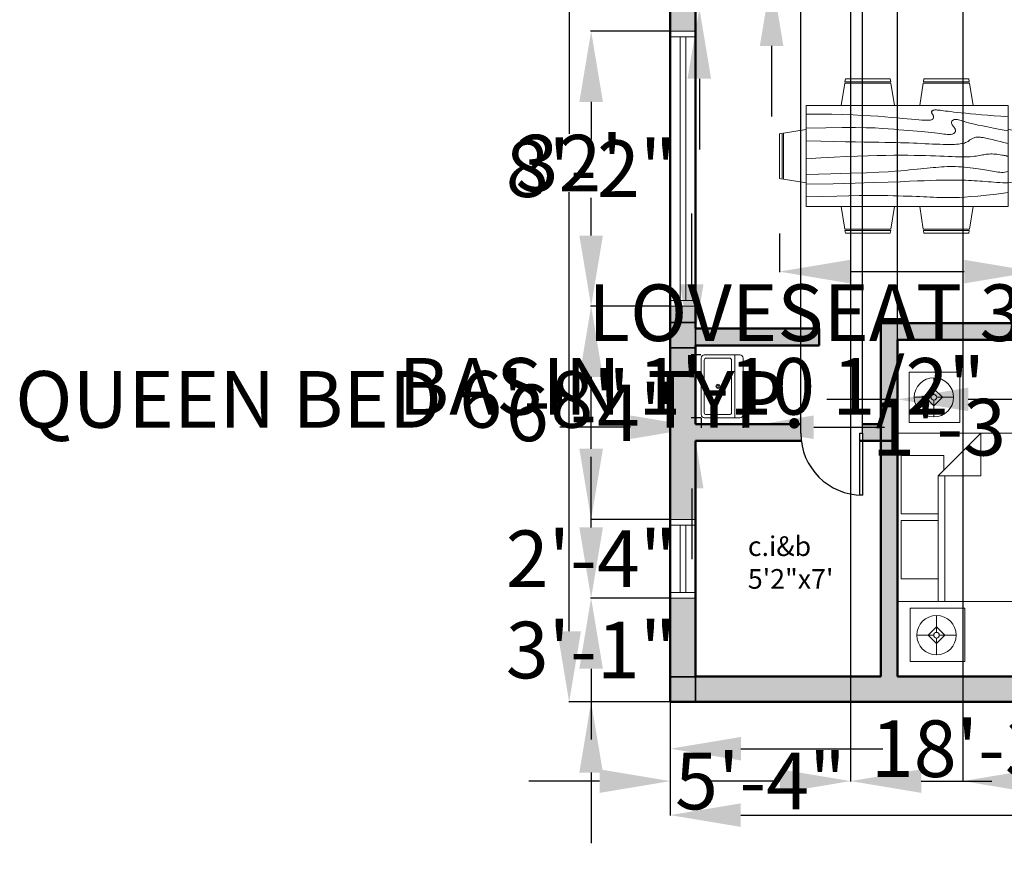
# Model space of a CAD drawing. Units: inches. Extents: x 25 to 82118, y 10 to 6494.
# Tile 1 of 9: x 40482 to 40833, y 3094 to 3391. Entities that reach past the tile are written whole.
import ezdxf

# ---------------------------------------------------------------- set-up
doc = ezdxf.new("R2010")
doc.units = ezdxf.units.IN
doc.header["$MEASUREMENT"] = 0
for name, color, linetype, lineweight in [('A-ANNO-DIMS', 2, 'Continuous', 18), ('A-AREA-IDEN', 7, 'Continuous', 25), ('A-DOOR', 3, 'Continuous', 25), ('A-FLOR-FIXT', 9, 'Continuous', 18), ('A-FURN', 8, 'Continuous', 18), ('A-GLAZ', 4, 'Continuous', 18), ('A-WALL', 7, 'Continuous', 50)]:
    doc.layers.add(name, color=color, linetype=linetype, lineweight=lineweight)
doc.layers.add('A-COLS', color=30, linetype='Continuous', lineweight=35, true_color=0xf26722)
doc.layers.add('A-WALL-PATT', color=18, linetype='Continuous', lineweight=13, true_color=0x000000)
doc.styles.get("Standard").update_dxf_attribs({"font": 'arial.ttf'})
doc.dimstyles.get("Standard").update_dxf_attribs({"dimtxt": 20.18, "dimasz": 25.18, "dimexe": 0.18, "dimexo": 0.0625, "dimgap": 0.09, "dimtad": 0, "dimtih": 1, "dimtoh": 1, "dimdec": 0, "dimzin": 0, "dimdsep": 46, "dimlunit": 3, "dimtxsty": 'Standard', "dimcen": 0.09, "dimadec": 0, "dimazin": 0, "dimtfac": 1, "dimtdec": 0, "dimtofl": 0, "dimtmove": 0, "dimatfit": 3, "dimfxl": 1, "dimtolj": 1, "dimtzin": 0, "dimarcsym": 0})

# ---------------------------------------------------------------- blocks, each defined once
blk = doc.blocks.new('Sink-single - 30 in top')
blk.add_line((-15, -3.999996), (15, -3.999996))
for points in [[(-13.5, 0), (13.5, 0)], [(-15, -18.499996), (-15, -1.5)], [(15, -1.5), (15, -18.499996)], [(-13.5, -17.499996), (-13.5, -6.499996)], [(-12.5, -5.499996), (12.5, -5.499996)], [(13.5, -6.499996), (13.5, -17.499996)], [(12.5, -18.499996), (-12.5, -18.499996)], [(13.5, -19.999996), (-13.5, -19.999996)]]:
    blk.add_lwpolyline(points)
for radius in [1, 0.5]:
    blk.add_circle((0, -11.999996), radius)
for centre, radius, start, end in [((-13.5, -1.5), 1.5, 90, 180), ((13.5, -1.5), 1.5, 0, 90), ((-12.5, -6.499996), 1, 90, 180), ((12.5, -6.499996), 1, 0, 90), ((-13.5, -18.499996), 1.5, 180, 270), ((-12.5, -17.499996), 1, 180, 270), ((12.5, -17.499996), 1, 270, 0), ((13.5, -18.499996), 1.5, 270, 0)]:
    blk.add_arc(centre, radius, start, end)
blk = doc.blocks.new('Bed - Queen')
for p, q in [((0, -80.00003), (0, 0)), ((0, 0), (59.99999, 0)), ((59.99999, 0), (59.99999, -80.00003)), ((7.99999, -1.2), (28.79998, -1.2)), ((7.99999, -14.4), (7.99999, -1.2)), ((28.79998, -1.2), (28.79998, -14.4)), ((31.19999, -1.2), (51.99999, -1.2)), ((31.19999, -14.4), (31.19999, -1.2)), ((51.99999, -1.2), (51.99999, -16.4)), ((0, -14.4), (44.8, -14.4)), ((44.8, -16.8), (0, -16.8)), ((59.99999, -29.6), (44.8, -14.4)), ((44.8, -14.4), (44.8, -29.6)), ((51.99999, -16.4), (46.79936, -16.4)), ((44.8, -29.6), (59.99999, -29.6)), ((59.99999, -80.00003), (0, -80.00003))]:
    blk.add_line(p, q)
blk = doc.blocks.new('Dining Set - 36 x 72 in.')
for p, q in [((-22.2343, 26.00059), (-23.4847, 17.99762)), ((-22.2304, 26), (-5.7608, 26)), ((-22, 27.5), (-22.1562, 26.50042)), ((-5.8416, 26.5), (-22.1534, 26.5)), ((-22, 27.5), (-6, 27.5)), ((-5.8437, 26.49966), (-6, 27.5)), ((-4.5152, 17.99762), (-5.7655, 25.99926)), ((5.7657, 26.00059), (4.5153, 17.99762)), ((5.7696, 26), (22.2392, 26)), ((6, 27.5), (5.8438, 26.50042)), ((22.1584, 26.5), (5.8466, 26.5)), ((6, 27.5), (22, 27.5)), ((22.1563, 26.49966), (22, 27.5)), ((23.4848, 17.99762), (22.2345, 25.99926)), ((36, 18), (-36, 18)), ((-36, 18), (-36, -18)), ((36, -18), (36, 18)), ((-45.5, 8), (-44.5004, 8.15617)), ((-45.5, 8), (-45.5, -8)), ((-44.5, -8.15843), (-44.5, 8.15338)), ((-44.0006, 8.23428), (-35.9976, 9.48474)), ((-44, 8.23041), (-44, -8.23915)), ((44.0006, 8.23428), (35.9976, 9.48474)), ((44, 8.23041), (44, -8.23915)), ((44.5, -8.15843), (44.5, 8.15338)), ((45.5, 8), (44.5005, 8.15617)), ((45.5, 8), (45.5, -8)), ((-44.4997, -8.15631), (-45.5, -8)), ((-35.9976, -9.48476), (-43.9993, -8.2345)), ((35.9976, -9.48476), (43.9993, -8.2345)), ((44.4997, -8.15631), (45.5, -8)), ((-36, -18), (36, -18)), ((-22.2343, -26.0006), (-23.4847, -17.99762)), ((-4.5152, -17.99762), (-5.7655, -25.99928)), ((5.7657, -26.0006), (4.5153, -17.99762)), ((23.4848, -17.99762), (22.2345, -25.99928)), ((-22.2304, -26), (-5.7608, -26)), ((-22, -27.5), (-22.1562, -26.50044)), ((-5.8416, -26.5), (-22.1534, -26.5)), ((-22, -27.5), (-6, -27.5)), ((-5.8437, -26.49967), (-6, -27.5)), ((5.7696, -26), (22.2392, -26)), ((6, -27.5), (5.8438, -26.50044)), ((22.1584, -26.5), (5.8466, -26.5)), ((6, -27.5), (22, -27.5)), ((22.1563, -26.49967), (22, -27.5))]:
    blk.add_line(p, q)
for points in [[(-36, 15), (-31.1772, 14.97754), (-26.8079, 14.91406), (-22.8538, 14.81543), (-19.276, 14.6875), (-16.0362, 14.53613), (-13.0957, 14.36718), (-10.4159, 14.18652), (-7.9583, 14), (-5.6904, 13.81315), (-3.6035, 13.63021), (-1.6954, 13.45508), (0.0365, 13.29166), (1.5945, 13.14388), (2.9811, 13.01562), (4.1988, 12.9108), (5.25, 12.83333), (6.1393, 12.78613), (6.8802, 12.76823), (7.4883, 12.77767), (7.9792, 12.8125), (8.3685, 12.87077), (8.6719, 12.95052), (8.9049, 13.0498), (9.0833, 13.16666), (9.2205, 13.29899), (9.3216, 13.44401), (9.3895, 13.59879), (9.4271, 13.76041), (9.4373, 13.92594), (9.4232, 14.09245), (9.3875, 14.257), (9.3333, 14.41666), (9.2638, 14.56917), (9.1836, 14.71484), (9.0975, 14.85465), (9.0104, 14.98958), (8.9272, 15.1206), (8.8529, 15.2487), (8.7922, 15.37483), (8.75, 15.5), (8.7305, 15.62467), (8.7344, 15.74739), (8.7617, 15.86621), (8.8125, 15.97916), (8.8867, 16.08431), (8.9844, 16.17968), (9.1055, 16.26334), (9.25, 16.33333), (9.4189, 16.38802), (9.6172, 16.42708), (9.8506, 16.45052), (10.125, 16.45833), (10.4463, 16.45052), (10.8203, 16.42708), (11.2529, 16.38802), (11.75, 16.33333), (12.3184, 16.26318), (12.9694, 16.17838), (13.7151, 16.07991), (14.5677, 15.96875), (15.5395, 15.84586), (16.6426, 15.71224), (17.8893, 15.56884), (19.2917, 15.41666), (20.859, 15.25667), (22.5879, 15.08984), (24.4721, 14.91715), (26.5052, 14.73958), (28.6809, 14.5581), (30.9929, 14.3737), (33.4347, 14.18733), (36, 14)], [(-36, 10), (-28.9766, 10.14274), (-23.1725, 10.20442), (-18.4241, 10.19775), (-14.5677, 10.13541), (-11.4399, 10.03011), (-8.877, 9.89453), (-6.7154, 9.74137), (-4.7917, 9.58333), (-2.9698, 9.43082), (-1.2246, 9.28515), (0.4415, 9.14534), (2.026, 9.01041), (3.5266, 8.87939), (4.9408, 8.7513), (6.266, 8.62516), (7.5, 8.5), (8.6411, 8.37549), (9.6914, 8.2539), (10.6538, 8.13818), (11.5312, 8.03125), (12.3267, 7.93603), (13.043, 7.85547), (13.6831, 7.79248), (14.25, 7.75), (14.7471, 7.7303), (15.1797, 7.73307), (15.5537, 7.75732), (15.875, 7.80208), (16.1494, 7.86637), (16.3828, 7.94922), (16.5811, 8.04964), (16.75, 8.16666), (16.8944, 8.29915), (17.0143, 8.44531), (17.1089, 8.60319), (17.1771, 8.77083), (17.218, 8.94629), (17.2305, 9.1276), (17.2137, 9.31282), (17.1667, 9.5), (17.0895, 9.6875), (16.987, 9.875), (16.8649, 10.0625), (16.7292, 10.25), (16.5856, 10.4375), (16.4401, 10.625), (16.2985, 10.8125), (16.1667, 11), (16.05, 11.18733), (15.9518, 11.3737), (15.8752, 11.5581), (15.8229, 11.73958), (15.798, 11.91715), (15.8034, 12.08984), (15.842, 12.25667), (15.9167, 12.41666), (16.0295, 12.56836), (16.1784, 12.70833), (16.3605, 12.83268), (16.5729, 12.9375), (16.8127, 13.01888), (17.0768, 13.07291), (17.3625, 13.0957), (17.6667, 13.08333), (17.9894, 13.03312), (18.3418, 12.94726), (18.7382, 12.82918), (19.1927, 12.68229), (19.7195, 12.51001), (20.3327, 12.31575), (21.0465, 12.10294), (21.875, 11.875), (22.8357, 11.63354), (23.959, 11.37304), (25.2786, 11.08618), (26.8282, 10.76562), (28.6414, 10.40405), (30.752, 9.99414), (33.1936, 9.52856), (36, 9)], [(-36, 5.5), (-30.7157, 5.3348), (-26.069, 5.20963), (-21.9946, 5.11767), (-18.4271, 5.05208), (-15.3009, 5.00602), (-12.5508, 4.97265), (-10.1112, 4.94515), (-7.9167, 4.91666), (-5.909, 4.88167), (-4.0586, 4.83984), (-2.3429, 4.79215), (-0.7396, 4.73958), (0.7739, 4.6831), (2.22, 4.6237), (3.6213, 4.56233), (5, 4.5), (6.373, 4.43782), (7.7344, 4.3776), (9.0723, 4.32129), (10.375, 4.27083), (11.6309, 4.22819), (12.8281, 4.19531), (13.9551, 4.17415), (15, 4.16666), (15.954, 4.17448), (16.819, 4.19791), (17.6001, 4.23698), (18.3021, 4.29166), (18.9299, 4.36198), (19.4883, 4.44791), (19.9823, 4.54948), (20.4167, 4.66666), (20.7969, 4.79899), (21.1302, 4.94401), (21.4245, 5.09879), (21.6875, 5.26041), (21.9271, 5.42594), (22.1511, 5.59245), (22.3672, 5.757), (22.5834, 5.91666), (22.8065, 6.06868), (23.0404, 6.21093), (23.2879, 6.34147), (23.5521, 6.45833), (23.8358, 6.55957), (24.142, 6.64323), (24.4735, 6.70735), (24.8334, 6.75), (25.2235, 6.76969), (25.642, 6.76692), (26.0858, 6.74267), (26.5521, 6.69791), (27.0379, 6.63362), (27.5404, 6.55078), (28.0565, 6.45036), (28.5834, 6.33333), (29.1242, 6.19987), (29.7071, 6.04687), (30.3661, 5.87044), (31.1354, 5.66666), (32.0493, 5.43164), (33.142, 5.16146), (34.4475, 4.85221), (36, 4.5)], [(-36, -1), (-30.7915, -0.6591), (-26.0195, -0.38216), (-21.6519, -0.16284), (-17.6563, 0.00521), (-14.0005, 0.12833), (-10.6523, 0.21289), (-7.5796, 0.26522), (-4.75, 0.29166), (-2.134, 0.29793), (0.2878, 0.28711), (2.5317, 0.26163), (4.6146, 0.22396), (6.5529, 0.17651), (8.3633, 0.12174), (10.0623, 0.06209), (11.6667, 0), (13.1899, -0.06201), (14.6341, -0.1211), (15.9982, -0.17432), (17.2813, -0.21875), (18.4823, -0.25147), (19.6003, -0.26953), (20.6343, -0.27002), (21.5834, -0.25), (22.4481, -0.20768), (23.2357, -0.14584), (23.9549, -0.06836), (24.6146, 0.02083), (25.2235, 0.11784), (25.7904, 0.21875), (26.3241, 0.31966), (26.8334, 0.41666), (27.3265, 0.50618), (27.8099, 0.58593), (28.2894, 0.65397), (28.7709, 0.70833), (29.2601, 0.74707), (29.763, 0.76823), (30.2855, 0.76985), (30.8334, 0.75), (31.4088, 0.70784), (31.9994, 0.64713), (32.589, 0.57275), (33.1615, 0.48958), (33.7008, 0.4025), (34.1908, 0.3164), (34.6153, 0.23616), (34.9584, 0.16666), (35.2099, 0.11165), (35.3848, 0.07031), (35.504, 0.04069), (35.5886, 0.02083), (35.6594, 0.00879), (35.7377, 0.0026), (35.8442, 0.00032), (36, 0)], [(-36, -6.5), (-27.1843, -6.31267), (-20.084, -6.1263), (-14.469, -5.9419), (-10.1094, -5.76042), (-6.7752, -5.58285), (-4.2363, -5.41016), (-2.2629, -5.24333), (-0.625, -5.08334), (0.8708, -4.93099), (2.2715, -4.78646), (3.5872, -4.64974), (4.8281, -4.52084), (6.0046, -4.39974), (7.127, -4.28646), (8.2053, -4.18099), (9.25, -4.08334), (10.2705, -3.99382), (11.2734, -3.91407), (12.2647, -3.84603), (13.25, -3.79167), (14.2354, -3.75293), (15.2266, -3.73177), (16.2295, -3.73015), (17.25, -3.75), (18.2912, -3.79248), (19.3451, -3.85547), (20.4009, -3.93604), (21.4479, -4.03125), (22.4754, -4.13819), (23.4727, -4.25391), (24.4289, -4.37549), (25.3334, -4.5), (26.1785, -4.62492), (26.9694, -4.74935), (27.7145, -4.87281), (28.4219, -4.99479), (29.1, -5.11483), (29.7572, -5.23242), (30.4016, -5.34709), (31.0417, -5.45834), (31.6837, -5.56437), (32.3262, -5.65821), (32.9658, -5.73153), (33.599, -5.77604), (34.2224, -5.78345), (34.8327, -5.74545), (35.4264, -5.65373), (36, -5.5)], [(-36, -10), (-26.4022, -9.81299), (-18.4675, -9.62891), (-11.9839, -9.45069), (-6.7396, -9.28125), (-2.5226, -9.12354), (0.8789, -8.98047), (3.6769, -8.85498), (6.0833, -8.75), (8.2767, -8.66765), (10.3021, -8.60677), (12.1712, -8.56543), (13.8958, -8.54167), (15.4876, -8.53353), (16.9583, -8.53907), (18.3197, -8.55632), (19.5834, -8.58334), (20.7616, -8.61841), (21.8685, -8.66081), (22.9188, -8.71004), (23.9271, -8.76563), (24.9081, -8.82707), (25.8763, -8.89388), (26.8465, -8.96558), (27.8334, -9.04167), (28.8474, -9.12118), (29.8828, -9.20117), (30.93, -9.27824), (31.9792, -9.34896), (33.0205, -9.40991), (34.0443, -9.45768), (35.0407, -9.48885), (36, -9.5)], [(-36, -14.5), (-30.0881, -14.33513), (-25.0332, -14.21224), (-20.7312, -14.12647), (-17.0781, -14.07292), (-13.97, -14.04671), (-11.3027, -14.04297), (-8.9724, -14.05681), (-6.875, -14.08334), (-4.9224, -14.11833), (-3.0905, -14.16016), (-1.3709, -14.20785), (0.2448, -14.26042), (1.7647, -14.3169), (3.1973, -14.3763), (4.5507, -14.43767), (5.8333, -14.5), (7.0554, -14.5621), (8.235, -14.62175), (9.3922, -14.67652), (10.5469, -14.72396), (11.7192, -14.76164), (12.929, -14.78711), (14.1965, -14.79794), (15.5417, -14.79167), (16.9933, -14.76424), (18.6152, -14.70508), (20.4804, -14.60197), (22.6615, -14.44271), (25.2312, -14.21509), (28.2624, -13.9069), (31.8277, -13.50594), (36, -13)]]:
    blk.add_lwpolyline(points)
blk = doc.blocks.new('Lamp - Table')
for p, q in [((0, 7), (0, 1)), ((-1, 0), (-7, 0)), ((0, 3), (-3, 0)), ((-3, 0), (0, -3)), ((3, 0), (0, 3)), ((0, -3), (3, 0)), ((1, 0), (7, 0)), ((0, -1), (0, -7))]:
    blk.add_line(p, q)
for radius in [7, 1]:
    blk.add_circle((0, 0), radius)
blk = doc.blocks.new('*U12')
for p, q in [((0, 0), (0, -6)), ((40, 0), (40, -6))]:
    blk.add_line(p, q)
blk.add_lwpolyline([(0, 0), (0, 40), (1.75, 40), (1.75, 0)], close=True)
blk.add_arc((0, 0), 40, 0, 90)
blk = doc.blocks.new('*D14')
at = {"layer": 'A-ANNO-DIMS', "color": 0, "lineweight": -2, "transparency": 16777216}
for p, q in [((40714.15, 3531.82), (40678.01, 3531.82)), ((40678.19, 3506.64), (40678.19, 3350.2)), ((40678.19, 3172.97), (40678.19, 3329.4)), ((40714.15, 3147.79), (40678.01, 3147.79))]:
    blk.add_line(p, q, dxfattribs=at)
at = {"layer": 'A-ANNO-DIMS', "color": 0, "transparency": 16777216}
for points in [[(40673.99, 3506.64), (40682.39, 3506.64), (40678.19, 3531.82)], [(40673.99, 3172.97), (40682.39, 3172.97), (40678.19, 3147.79)]]:
    blk.add_solid(points, dxfattribs=at)
at = {"layer": 'Defpoints', "color": 0, "transparency": 16777216}
for p in [(40714.21, 3531.82), (40678.19, 3147.79), (40714.21, 3147.79)]:
    blk.add_point(p, dxfattribs=at)
at = {"layer": 'A-ANNO-DIMS', "color": 0, "transparency": 16777216, "insert": (40678.19, 3339.8), "char_height": 20.18, "attachment_point": 5}
blk.add_mtext("\\A1;32'", dxfattribs=at)
blk = doc.blocks.new('*D18')
at = {"layer": 'A-ANNO-DIMS', "color": 0, "lineweight": -2, "transparency": 16777216}
for p, q in [((40714.15, 3147.72), (40714.15, 3107.28)), ((41074.21, 3147.76), (41074.21, 3107.28)), ((40739.33, 3107.46), (40876.97, 3107.46)), ((41049.03, 3107.46), (40911.38, 3107.46))]:
    blk.add_line(p, q, dxfattribs=at)
at = {"layer": 'A-ANNO-DIMS', "color": 0, "transparency": 16777216}
for points in [[(40739.33, 3111.65), (40739.33, 3103.26), (40714.15, 3107.46)], [(41049.03, 3111.65), (41049.03, 3103.26), (41074.21, 3107.46)]]:
    blk.add_solid(points, dxfattribs=at)
at = {"layer": 'Defpoints', "color": 0, "transparency": 16777216}
for p in [(40714.15, 3147.79), (41074.21, 3147.82), (41074.21, 3107.46)]:
    blk.add_point(p, dxfattribs=at)
at = {"layer": 'A-ANNO-DIMS', "color": 0, "transparency": 16777216, "insert": (40894.18, 3107.46), "char_height": 20.18, "attachment_point": 5}
blk.add_mtext("\\A1;30'", dxfattribs=at)
blk = doc.blocks.new('*D20')
at = {"layer": 'A-ANNO-DIMS', "color": 0, "lineweight": -2, "transparency": 16777216}
for p, q in [((40714.21, 3147.72), (40714.21, 3130.95)), ((40933.21, 3147.72), (40933.21, 3130.95)), ((40739.39, 3131.13), (40789.91, 3131.13)), ((40908.03, 3131.13), (40857.51, 3131.13))]:
    blk.add_line(p, q, dxfattribs=at)
at = {"layer": 'A-ANNO-DIMS', "color": 0, "transparency": 16777216}
for points in [[(40739.39, 3135.32), (40739.39, 3126.93), (40714.21, 3131.13)], [(40908.03, 3135.32), (40908.03, 3126.93), (40933.21, 3131.13)]]:
    blk.add_solid(points, dxfattribs=at)
at = {"layer": 'Defpoints', "color": 0, "transparency": 16777216}
for p in [(40714.21, 3147.79), (40933.21, 3147.79), (40933.21, 3131.13)]:
    blk.add_point(p, dxfattribs=at)
at = {"layer": 'A-ANNO-DIMS', "color": 0, "transparency": 16777216, "insert": (40823.71, 3131.13), "char_height": 20.18, "attachment_point": 5}
blk.add_mtext('\\A1;18\'-3"', dxfattribs=at)
blk = doc.blocks.new('COL-9X9')
h = blk.add_hatch(color=256)
h.dxf.hatch_style = 1
h.paths.add_polyline_path([(9, 9), (0, 9), (0, 0), (9, 0)])
blk.add_lwpolyline([(0, 0), (9, 0), (9, 9), (0, 9)], close=True)
blk = doc.blocks.new('*D25')
at = {"layer": 'A-ANNO-DIMS', "color": 0, "lineweight": -2, "transparency": 16777216}
for p, q in [((40724.56, 3429.21), (40724.56, 3454.39)), ((40724.56, 3454.39), (40749.74, 3454.39)), ((40723.27, 3404.03), (40724.74, 3404.03)), ((40723.27, 3395.03), (40724.74, 3395.03)), ((40724.56, 3369.85), (40724.56, 3344.67))]:
    blk.add_line(p, q, dxfattribs=at)
at = {"layer": 'A-ANNO-DIMS', "color": 0, "transparency": 16777216}
for points in [[(40720.36, 3429.21), (40728.76, 3429.21), (40724.56, 3404.03)], [(40720.36, 3369.85), (40728.76, 3369.85), (40724.56, 3395.03)]]:
    blk.add_solid(points, dxfattribs=at)
at = {"layer": 'Defpoints', "color": 0, "transparency": 16777216}
for p in [(40723.21, 3404.03), (40724.56, 3404.03), (40723.21, 3395.03)]:
    blk.add_point(p, dxfattribs=at)
at = {"layer": 'A-ANNO-DIMS', "color": 0, "transparency": 16777216, "insert": (40876.22, 3454.39), "char_height": 20.18, "attachment_point": 5}
blk.add_mtext('\\A1;COLUMN 0\'-9" TYP.', dxfattribs=at)
blk = doc.blocks.new('*D26')
at = {"layer": 'A-ANNO-DIMS', "color": 0, "lineweight": -2, "transparency": 16777216}
for p, q in [((40689.03, 3405.38), (40663.85, 3405.38)), ((40714.21, 3404.09), (40714.21, 3405.56)), ((40723.21, 3404.09), (40723.21, 3405.56)), ((40748.39, 3405.38), (40773.57, 3405.38))]:
    blk.add_line(p, q, dxfattribs=at)
at = {"layer": 'A-ANNO-DIMS', "color": 0, "transparency": 16777216}
for points in [[(40689.03, 3409.57), (40689.03, 3401.18), (40714.21, 3405.38)], [(40748.39, 3409.57), (40748.39, 3401.18), (40723.21, 3405.38)]]:
    blk.add_solid(points, dxfattribs=at)
at = {"layer": 'Defpoints', "color": 0, "transparency": 16777216}
for p in [(40714.21, 3405.38), (40714.21, 3404.03), (40723.21, 3404.03)]:
    blk.add_point(p, dxfattribs=at)
at = {"layer": 'A-ANNO-DIMS', "color": 0, "transparency": 16777216, "insert": (40602.26, 3405.38), "char_height": 20.18, "attachment_point": 5}
blk.add_mtext('\\A1;0\'-9" TYP.', dxfattribs=at)
blk = doc.blocks.new('*D35')
at = {"layer": 'A-ANNO-DIMS', "color": 0, "lineweight": -2, "transparency": 16777216}
for p, q in [((40795.21, 3255.62), (40770.03, 3255.62)), ((40795.21, 3243.68), (40795.21, 3255.8)), ((40850.03, 3255.62), (40820.39, 3255.62)), ((40875.21, 3243.68), (40875.21, 3255.8))]:
    blk.add_line(p, q, dxfattribs=at)
at = {"layer": 'A-ANNO-DIMS', "color": 0, "transparency": 16777216}
for points in [[(40820.39, 3259.82), (40820.39, 3251.42), (40795.21, 3255.62)], [(40850.03, 3259.82), (40850.03, 3251.42), (40875.21, 3255.62)]]:
    blk.add_solid(points, dxfattribs=at)
at = {"layer": 'Defpoints', "color": 0, "transparency": 16777216}
for p in [(40795.21, 3255.62), (40795.21, 3243.62), (40875.21, 3243.62)]:
    blk.add_point(p, dxfattribs=at)
at = {"layer": 'A-ANNO-DIMS', "color": 0, "transparency": 16777216, "insert": (40621.51, 3255.62), "char_height": 20.18, "attachment_point": 5}
blk.add_mtext('\\A1;QUEEN BED 6\'-8" TYP.', dxfattribs=at)
blk = doc.blocks.new('*D41')
at = {"layer": 'A-ANNO-DIMS', "color": 0, "lineweight": -2, "transparency": 16777216}
for p, q in [((40721.85, 3296.64), (40721.85, 3321.82)), ((40725.15, 3271.46), (40721.67, 3271.46)), ((40725.15, 3249.06), (40721.67, 3249.06)), ((40721.85, 3223.88), (40721.85, 3198.7))]:
    blk.add_line(p, q, dxfattribs=at)
at = {"layer": 'A-ANNO-DIMS', "color": 0, "transparency": 16777216}
for points in [[(40717.65, 3296.64), (40726.05, 3296.64), (40721.85, 3271.46)], [(40717.65, 3223.88), (40726.05, 3223.88), (40721.85, 3249.06)]]:
    blk.add_solid(points, dxfattribs=at)
at = {"layer": 'Defpoints', "color": 0, "transparency": 16777216}
for p in [(40725.21, 3271.46), (40721.85, 3249.06), (40725.21, 3249.06)]:
    blk.add_point(p, dxfattribs=at)
at = {"layer": 'A-ANNO-DIMS', "color": 0, "transparency": 16777216, "insert": (40721.85, 3260.26), "char_height": 20.18, "attachment_point": 5}
blk.add_mtext('\\A1;BASIN 1\'-10 1/2"', dxfattribs=at)
blk = doc.blocks.new('*D42')
at = {"layer": 'A-ANNO-DIMS', "color": 0, "lineweight": -2, "transparency": 16777216}
for p, q in [((40725.21, 3248.99), (40725.21, 3245.52)), ((40740.15, 3248.99), (40740.15, 3245.52)), ((40700.03, 3245.7), (40674.85, 3245.7)), ((40765.33, 3245.7), (40790.51, 3245.7))]:
    blk.add_line(p, q, dxfattribs=at)
at = {"layer": 'A-ANNO-DIMS', "color": 0, "transparency": 16777216}
for points in [[(40700.03, 3249.89), (40700.03, 3241.5), (40725.21, 3245.7)], [(40765.33, 3249.89), (40765.33, 3241.5), (40740.15, 3245.7)]]:
    blk.add_solid(points, dxfattribs=at)
at = {"layer": 'Defpoints', "color": 0, "transparency": 16777216}
for p in [(40725.21, 3249.06), (40740.15, 3249.06), (40740.15, 3245.7)]:
    blk.add_point(p, dxfattribs=at)
at = {"layer": 'A-ANNO-DIMS', "color": 0, "transparency": 16777216, "insert": (40816.47, 3245.7), "char_height": 20.18, "attachment_point": 5}
blk.add_mtext('\\A1;1\'-3"', dxfattribs=at)
blk = doc.blocks.new('*D47')
at = {"layer": 'A-ANNO-DIMS', "color": 0, "lineweight": -2, "transparency": 16777216}
for p, q in [((40753.09, 3314.74), (40753.09, 3300.97)), ((40844.09, 3314.74), (40844.09, 3300.97)), ((40778.27, 3301.15), (40818.91, 3301.15)), ((40844.09, 3301.15), (40869.27, 3301.15))]:
    blk.add_line(p, q, dxfattribs=at)
at = {"layer": 'A-ANNO-DIMS', "color": 0, "transparency": 16777216}
for points in [[(40778.27, 3305.35), (40778.27, 3296.95), (40753.09, 3301.15)], [(40818.91, 3305.35), (40818.91, 3296.95), (40844.09, 3301.15)]]:
    blk.add_solid(points, dxfattribs=at)
at = {"layer": 'Defpoints', "color": 0, "transparency": 16777216}
for p in [(40753.09, 3314.8), (40844.09, 3314.8), (40844.09, 3301.15)]:
    blk.add_point(p, dxfattribs=at)
at = {"layer": 'A-ANNO-DIMS', "color": 0, "transparency": 16777216, "insert": (40980.26, 3301.15), "char_height": 20.18, "attachment_point": 5}
blk.add_mtext('\\A1;DINING SET 7\'-7"', dxfattribs=at)
blk = doc.blocks.new('*D49')
at = {"layer": 'A-ANNO-DIMS', "color": 0, "lineweight": -2, "transparency": 16777216}
for p, q in [((40962.31, 3286.49), (40937.13, 3286.49)), ((40987.49, 3280.33), (40987.49, 3286.67)), ((41028.96, 3280.33), (41028.96, 3286.67)), ((41054.14, 3286.49), (41079.32, 3286.49))]:
    blk.add_line(p, q, dxfattribs=at)
at = {"layer": 'A-ANNO-DIMS', "color": 0, "transparency": 16777216}
for points in [[(40962.31, 3290.68), (40962.31, 3282.29), (40987.49, 3286.49)], [(41054.14, 3290.68), (41054.14, 3282.29), (41028.96, 3286.49)]]:
    blk.add_solid(points, dxfattribs=at)
at = {"layer": 'Defpoints', "color": 0, "transparency": 16777216}
for p in [(40987.49, 3286.49), (40987.49, 3280.26), (41028.96, 3280.26)]:
    blk.add_point(p, dxfattribs=at)
at = {"layer": 'A-ANNO-DIMS', "color": 0, "transparency": 16777216, "insert": (40808.81, 3286.49), "char_height": 20.18, "attachment_point": 5}
blk.add_mtext('\\A1;LOVESEAT 3\'-5 1/2"', dxfattribs=at)
blk = doc.blocks.new('*D51')
at = {"layer": 'A-ANNO-DIMS', "color": 0, "lineweight": -2, "transparency": 16777216}
for p, q in [((40750.31, 3454.92), (40750.31, 3480.1)), ((40746.92, 3429.74), (40750.49, 3429.74)), ((40746.92, 3406.76), (40750.49, 3406.76)), ((40750.31, 3381.58), (40750.31, 3356.4))]:
    blk.add_line(p, q, dxfattribs=at)
at = {"layer": 'A-ANNO-DIMS', "color": 0, "transparency": 16777216}
for points in [[(40746.11, 3454.92), (40754.5, 3454.92), (40750.31, 3429.74)], [(40746.11, 3381.58), (40754.5, 3381.58), (40750.31, 3406.76)]]:
    blk.add_solid(points, dxfattribs=at)
at = {"layer": 'Defpoints', "color": 0, "transparency": 16777216}
for p in [(40746.86, 3429.74), (40750.31, 3429.74), (40746.86, 3406.76)]:
    blk.add_point(p, dxfattribs=at)
at = {"layer": 'A-ANNO-DIMS', "color": 0, "transparency": 16777216, "insert": (40750.31, 3418.25), "char_height": 20.18, "attachment_point": 5}
blk.add_mtext('\\A1;FRIDGE 1\'-11"', dxfattribs=at)
blk = doc.blocks.new('*D56')
at = {"layer": 'A-ANNO-DIMS', "color": 0, "lineweight": -2, "transparency": 16777216}
for p, q in [((40778.43, 3531.76), (40778.43, 3119.41)), ((40818.43, 3531.76), (40818.43, 3119.41)), ((40753.25, 3119.59), (40728.07, 3119.59)), ((40843.61, 3119.59), (40868.79, 3119.59))]:
    blk.add_line(p, q, dxfattribs=at)
at = {"layer": 'A-ANNO-DIMS', "color": 0, "transparency": 16777216}
for points in [[(40753.25, 3123.78), (40753.25, 3115.39), (40778.43, 3119.59)], [(40843.61, 3123.78), (40843.61, 3115.39), (40818.43, 3119.59)]]:
    blk.add_solid(points, dxfattribs=at)
at = {"layer": 'Defpoints', "color": 0, "transparency": 16777216}
for p in [(40778.43, 3531.82), (40818.43, 3531.82), (40818.43, 3119.59)]:
    blk.add_point(p, dxfattribs=at)
at = {"layer": 'A-ANNO-DIMS', "color": 0, "transparency": 16777216, "insert": (40895.69, 3119.59), "char_height": 20.18, "attachment_point": 5}
blk.add_mtext('\\A1;3\'-4"', dxfattribs=at)
blk = doc.blocks.new('*D57')
at = {"layer": 'A-ANNO-DIMS', "color": 0, "lineweight": -2, "transparency": 16777216}
for p, q in [((40714.21, 3531.76), (40714.21, 3119.41)), ((40778.43, 3531.76), (40778.43, 3119.41)), ((40689.03, 3119.59), (40663.85, 3119.59)), ((40803.61, 3119.59), (40828.79, 3119.59))]:
    blk.add_line(p, q, dxfattribs=at)
at = {"layer": 'A-ANNO-DIMS', "color": 0, "transparency": 16777216}
for points in [[(40689.03, 3123.78), (40689.03, 3115.39), (40714.21, 3119.59)], [(40803.61, 3123.78), (40803.61, 3115.39), (40778.43, 3119.59)]]:
    blk.add_solid(points, dxfattribs=at)
at = {"layer": 'Defpoints', "color": 0, "transparency": 16777216}
for p in [(40714.21, 3531.82), (40778.43, 3531.82), (40778.43, 3119.59)]:
    blk.add_point(p, dxfattribs=at)
at = {"layer": 'A-ANNO-DIMS', "color": 0, "transparency": 16777216, "insert": (40746.32, 3119.59), "char_height": 20.18, "attachment_point": 5}
blk.add_mtext('\\A1;5\'-4"', dxfattribs=at)
blk = doc.blocks.new('*D58')
at = {"layer": 'A-ANNO-DIMS', "color": 0, "lineweight": -2, "transparency": 16777216}
for p, q in [((40735.53, 3572.85), (40710.35, 3572.85)), ((40760.71, 3246.88), (40760.71, 3573.03)), ((40782.73, 3246.88), (40782.73, 3573.03)), ((40807.91, 3572.85), (40833.09, 3572.85))]:
    blk.add_line(p, q, dxfattribs=at)
at = {"layer": 'A-ANNO-DIMS', "color": 0, "transparency": 16777216}
for points in [[(40735.53, 3577.05), (40735.53, 3568.66), (40760.71, 3572.85)], [(40807.91, 3577.05), (40807.91, 3568.66), (40782.73, 3572.85)]]:
    blk.add_solid(points, dxfattribs=at)
at = {"layer": 'Defpoints', "color": 0, "transparency": 16777216}
for p in [(40782.73, 3572.85), (40760.71, 3246.82), (40782.73, 3246.82)]:
    blk.add_point(p, dxfattribs=at)
at = {"layer": 'A-ANNO-DIMS', "color": 0, "transparency": 16777216, "insert": (40866.89, 3572.85), "char_height": 20.18, "attachment_point": 5}
blk.add_mtext('\\A1;1\'-10"', dxfattribs=at)
blk = doc.blocks.new('*D59')
at = {"layer": 'A-ANNO-DIMS', "color": 0, "lineweight": -2, "transparency": 16777216}
for p, q in [((40686.01, 3210), (40686.01, 3235.18)), ((40714.15, 3184.82), (40685.83, 3184.82)), ((40714.15, 3147.79), (40685.83, 3147.79)), ((40686.01, 3122.61), (40686.01, 3097.43))]:
    blk.add_line(p, q, dxfattribs=at)
at = {"layer": 'A-ANNO-DIMS', "color": 0, "transparency": 16777216}
for points in [[(40681.81, 3210), (40690.21, 3210), (40686.01, 3184.82)], [(40681.81, 3122.61), (40690.21, 3122.61), (40686.01, 3147.79)]]:
    blk.add_solid(points, dxfattribs=at)
at = {"layer": 'Defpoints', "color": 0, "transparency": 16777216}
for p in [(40686.01, 3184.82), (40714.21, 3184.82), (40714.21, 3147.79)]:
    blk.add_point(p, dxfattribs=at)
at = {"layer": 'A-ANNO-DIMS', "color": 0, "transparency": 16777216, "insert": (40686.01, 3166.3), "char_height": 20.18, "attachment_point": 5}
blk.add_mtext('\\A1;3\'-1"', dxfattribs=at)
blk = doc.blocks.new('*D60')
at = {"layer": 'A-ANNO-DIMS', "color": 0, "lineweight": -2, "transparency": 16777216}
for p, q in [((40686.01, 3238), (40686.01, 3263.18)), ((40714.15, 3212.82), (40685.83, 3212.82)), ((40714.15, 3184.82), (40685.83, 3184.82)), ((40686.01, 3159.64), (40686.01, 3134.46))]:
    blk.add_line(p, q, dxfattribs=at)
at = {"layer": 'A-ANNO-DIMS', "color": 0, "transparency": 16777216}
for points in [[(40681.81, 3238), (40690.21, 3238), (40686.01, 3212.82)], [(40681.81, 3159.64), (40690.21, 3159.64), (40686.01, 3184.82)]]:
    blk.add_solid(points, dxfattribs=at)
at = {"layer": 'Defpoints', "color": 0, "transparency": 16777216}
for p in [(40686.01, 3212.82), (40714.21, 3212.82), (40714.21, 3184.82)]:
    blk.add_point(p, dxfattribs=at)
at = {"layer": 'A-ANNO-DIMS', "color": 0, "transparency": 16777216, "insert": (40686.01, 3198.82), "char_height": 20.18, "attachment_point": 5}
blk.add_mtext('\\A1;2\'-4"', dxfattribs=at)
blk = doc.blocks.new('*D61')
at = {"layer": 'A-ANNO-DIMS', "color": 0, "lineweight": -2, "transparency": 16777216}
for p, q in [((40714.15, 3288.82), (40685.83, 3288.82)), ((40686.01, 3263.64), (40686.01, 3261.21)), ((40686.01, 3238), (40686.01, 3240.43)), ((40714.15, 3212.82), (40685.83, 3212.82))]:
    blk.add_line(p, q, dxfattribs=at)
at = {"layer": 'A-ANNO-DIMS', "color": 0, "transparency": 16777216}
for points in [[(40681.81, 3263.64), (40690.21, 3263.64), (40686.01, 3288.82)], [(40681.81, 3238), (40690.21, 3238), (40686.01, 3212.82)]]:
    blk.add_solid(points, dxfattribs=at)
at = {"layer": 'Defpoints', "color": 0, "transparency": 16777216}
for p in [(40686.01, 3288.82), (40714.21, 3288.82), (40714.21, 3212.82)]:
    blk.add_point(p, dxfattribs=at)
at = {"layer": 'A-ANNO-DIMS', "color": 0, "transparency": 16777216, "insert": (40686.01, 3250.82), "char_height": 20.18, "attachment_point": 5}
blk.add_mtext('\\A1;6\'-4"', dxfattribs=at)
blk = doc.blocks.new('*D62')
at = {"layer": 'A-ANNO-DIMS', "color": 0, "lineweight": -2, "transparency": 16777216}
for p, q in [((40714.15, 3386.82), (40685.83, 3386.82)), ((40686.01, 3361.64), (40686.01, 3348.21)), ((40686.01, 3314), (40686.01, 3327.43)), ((40714.15, 3288.82), (40685.83, 3288.82))]:
    blk.add_line(p, q, dxfattribs=at)
at = {"layer": 'A-ANNO-DIMS', "color": 0, "transparency": 16777216}
for points in [[(40681.81, 3361.64), (40690.21, 3361.64), (40686.01, 3386.82)], [(40681.81, 3314), (40690.21, 3314), (40686.01, 3288.82)]]:
    blk.add_solid(points, dxfattribs=at)
at = {"layer": 'Defpoints', "color": 0, "transparency": 16777216}
for p in [(40686.01, 3386.82), (40714.21, 3386.82), (40714.21, 3288.82)]:
    blk.add_point(p, dxfattribs=at)
at = {"layer": 'A-ANNO-DIMS', "color": 0, "transparency": 16777216, "insert": (40686.01, 3337.82), "char_height": 20.18, "attachment_point": 5}
blk.add_mtext('\\A1;8\'-2"', dxfattribs=at)
blk = doc.blocks.new('*D67')
at = {"layer": 'A-ANNO-DIMS', "color": 0, "lineweight": -2, "transparency": 16777216}
for p, q in [((40770.03, 3572.85), (40744.85, 3572.85)), ((40795.21, 3156.88), (40795.21, 3573.03)), ((40838.63, 3156.88), (40838.63, 3573.03)), ((40863.81, 3572.85), (40888.99, 3572.85))]:
    blk.add_line(p, q, dxfattribs=at)
at = {"layer": 'A-ANNO-DIMS', "color": 0, "transparency": 16777216}
for points in [[(40770.03, 3577.05), (40770.03, 3568.66), (40795.21, 3572.85)], [(40863.81, 3577.05), (40863.81, 3568.66), (40838.63, 3572.85)]]:
    blk.add_solid(points, dxfattribs=at)
at = {"layer": 'Defpoints', "color": 0, "transparency": 16777216}
for p in [(40838.63, 3572.85), (40795.21, 3156.82), (40838.63, 3156.82)]:
    blk.add_point(p, dxfattribs=at)
at = {"layer": 'A-ANNO-DIMS', "color": 0, "transparency": 16777216, "insert": (40939.41, 3572.85), "char_height": 20.18, "attachment_point": 5}
blk.add_mtext('\\A1;3\'-7 1/2"', dxfattribs=at)

msp = doc.modelspace()

# ---------------------------------------------------------------- hatches: boundary and pattern name
at = {"layer": 'A-WALL-PATT'}
h = msp.add_hatch(color=256, dxfattribs=at)
h.dxf.hatch_style = 1
h.paths.add_polyline_path([(40778.43, 3531.82), (40723.21, 3531.82), (40723.21, 3522.82), (40778.54, 3522.82, -0.01877), (40778.43, 3525.82)])
h.paths.add_polyline_path([(40723.21, 3522.82), (40714.21, 3522.82), (40714.21, 3500.82), (40723.21, 3500.82)])
h.paths.add_polyline_path([(40723.21, 3424.82), (40714.21, 3424.82), (40714.21, 3404.03), (40723.21, 3404.03)])
h.paths.add_polyline_path([(40723.21, 3395.03), (40714.21, 3395.03), (40714.21, 3386.82), (40723.21, 3386.82)])
h.paths.add_polyline_path([(40901.65, 3531.82), (40834.16, 3531.82), (40834.16, 3522.82), (40901.65, 3522.82)])
h.paths.add_polyline_path([(40825.16, 3531.82), (40818.43, 3531.82), (40818.43, 3525.82), (40818.43, 3522.82), (40825.16, 3522.82)])
h.paths.add_polyline_path([(40961.21, 3531.82), (40910.65, 3531.82), (40910.65, 3522.82), (40961.21, 3522.82)])
h.paths.add_polyline_path([(41065.21, 3531.82), (41013.21, 3531.82), (41013.21, 3522.82), (41065.21, 3522.82)])
h.paths.add_polyline_path([(41074.21, 3522.82), (41065.21, 3522.82), (41065.21, 3506.52), (41074.21, 3506.52)])
h.paths.add_polyline_path([(41074.21, 3430.52), (41065.21, 3430.52), (41065.21, 3428.74), (41065.21, 3380.62), (41074.21, 3380.62)])
h.paths.add_polyline_path([(41074.21, 3371.62), (41065.21, 3371.62), (41065.21, 3355.41), (41074.21, 3355.41)])
h.paths.add_polyline_path([(41065.36, 3378.82), (40909.21, 3378.82), (40909.21, 3382.1), (40903.21, 3382.1), (40903.21, 3372.82), (41065.36, 3372.82)])
h.paths.add_polyline_path([(40933.21, 3372.82), (40927.21, 3372.82), (40927.21, 3282.62), (40933.21, 3282.62)])
h.paths.add_polyline_path([(41074.21, 3279.41), (41065.21, 3279.41), (41065.21, 3240.82), (41074.21, 3240.82)])
h.paths.add_polyline_path([(41065.21, 3246.82), (41052.05, 3246.82), (41052.05, 3240.82), (41065.21, 3240.82)])
h.paths.add_polyline_path([(40985.75, 3202.89), (41023.1, 3202.89), (41023.1, 3229.01), (40985.75, 3229.01)], flags=9)
h.paths.add_polyline_path([(40960.75, 3302.54), (40998.1, 3302.54), (40998.1, 3328.66), (40960.75, 3328.66)], flags=9)
h = msp.add_hatch(color=256, dxfattribs=at)
h.dxf.hatch_style = 1
h.paths.add_polyline_path([(40784.59, 3402.82), (40723.21, 3402.82), (40723.21, 3396.82), (40784.59, 3396.82)])
h.paths.add_polyline_path([(40833.21, 3522.82), (40827.21, 3522.82), (40827.21, 3402.75), (40830.71, 3402.75), (40830.71, 3396.82), (40833.21, 3396.82)])
h.paths.add_polyline_path([(40767.21, 3280.82), (40723.21, 3280.82), (40723.21, 3274.82), (40767.21, 3274.82)])
h.paths.add_polyline_path([(40723.21, 3288.82), (40714.21, 3288.82), (40714.21, 3283), (40723.21, 3283)])
h = msp.add_hatch(color=256, dxfattribs=at)
h.dxf.hatch_style = 1
h.paths.add_polyline_path([(40723.21, 3274), (40714.21, 3274), (40714.21, 3212.82), (40723.21, 3212.82), (40723.21, 3240.82), (40760.88, 3240.82, -0.030698), (40760.71, 3243.52), (40760.71, 3246.82), (40723.21, 3246.82)])
h.paths.add_polyline_path([(40789.21, 3246.82), (40782.73, 3246.82), (40782.73, 3243.52), (40782.73, 3240.82), (40789.21, 3240.82)])
h.paths.add_polyline_path([(40795.21, 3276.82), (40880.67, 3276.82), (40880.67, 3282.82), (40789.21, 3282.82), (40789.21, 3240.82), (40795.21, 3240.82), (40795.21, 3243.62)])
h.paths.add_polyline_path([(40795.21, 3240.82), (40789.21, 3240.82), (40789.21, 3156.82), (40723.21, 3156.82), (40723.21, 3147.82), (40838.63, 3147.82), (40838.63, 3156.82), (40795.21, 3156.82)])
h.paths.add_polyline_path([(40723.21, 3184.82), (40714.21, 3184.82), (40714.21, 3156.79), (40723.21, 3156.79), (40723.21, 3156.82)])
h.paths.add_polyline_path([(40924.06, 3156.82), (40890.63, 3156.82), (40890.63, 3147.82), (40924.06, 3147.82)])
h.paths.add_polyline_path([(40933.21, 3240.82), (40937.89, 3240.82), (40937.89, 3246.82), (40933.21, 3246.82), (40933.21, 3276.82), (40927.21, 3276.82), (40927.21, 3156.82), (40933.21, 3156.82)])
h.paths.add_polyline_path([(41000.05, 3246.82), (40977.89, 3246.82), (40977.89, 3240.82), (41000.05, 3240.82)])

# ---------------------------------------------------------------- linework, layer by layer
at = {"layer": 'A-FURN'}
for points in [[(40799.33, 3265.37), (40817.38, 3265.37), (40817.38, 3247.34), (40799.33, 3247.34)], [(40799.7, 3181.27), (40819.16, 3181.27), (40819.16, 3162.23), (40799.7, 3162.23)]]:
    msp.add_lwpolyline(points, close=True, dxfattribs=at)
at = {"layer": 'A-GLAZ'}
for p, q in [((40723.21, 3386.82), (40714.21, 3386.82)), ((40723.21, 3384.82), (40714.21, 3384.82)), ((40717.71, 3384.82), (40717.71, 3290.82)), ((40719.71, 3384.82), (40719.71, 3290.82)), ((40723.21, 3290.82), (40714.21, 3290.82)), ((40723.21, 3288.82), (40714.21, 3288.82)), ((40723.21, 3212.82), (40714.21, 3212.82)), ((40723.21, 3210.82), (40714.21, 3210.82)), ((40717.71, 3210.82), (40717.71, 3186.82)), ((40719.71, 3210.82), (40719.71, 3186.82)), ((40723.21, 3186.82), (40714.21, 3186.82)), ((40723.21, 3184.82), (40714.21, 3184.82))]:
    msp.add_line(p, q, dxfattribs=at)
at = {"layer": 'A-WALL'}
for p, q in [((40714.21, 3147.82), (40714.21, 3531.82)), ((40723.21, 3280.82), (40723.21, 3396.82)), ((40723.21, 3280.82), (40767.21, 3280.82)), ((40767.21, 3274.82), (40767.21, 3280.82)), ((40789.21, 3282.82), (40789.21, 3156.82)), ((40880.67, 3282.82), (40789.21, 3282.82)), ((40795.21, 3276.82), (40795.21, 3156.82)), ((40880.67, 3276.82), (40795.21, 3276.82)), ((40723.21, 3274.82), (40767.21, 3274.82)), ((40723.21, 3246.82), (40723.21, 3274.82)), ((40760.71, 3246.82), (40723.21, 3246.82)), ((40789.21, 3246.82), (40782.73, 3246.82)), ((40723.21, 3156.82), (40723.21, 3240.82)), ((40760.88, 3240.82), (40723.21, 3240.82)), ((40795.21, 3240.82), (40781.77, 3240.82)), ((40789.21, 3156.82), (40723.21, 3156.82)), ((40927.21, 3156.82), (40795.21, 3156.82)), ((41074.21, 3147.82), (40714.21, 3147.82))]:
    msp.add_line(p, q, dxfattribs=at)

# ---------------------------------------------------------------- block references
at = {"layer": 'A-COLS', "rotation": 89.99999999991314}
for p in [(40723.21, 3274), (40723.21, 3147.79)]:
    msp.add_blockref('COL-9X9', p, dxfattribs=at)
at = {"layer": 'A-DOOR', "xscale": 0.5505718407670358, "yscale": 0.5505718407670358, "zscale": 0.5505718407670358, "rotation": 180}
msp.add_blockref('*U12', (40782.73, 3243.52), dxfattribs=at)
at = {"layer": 'A-FLOR-FIXT', "xscale": 0.7467501646834624, "yscale": 0.7467501646834624, "zscale": 0.7467501646834624, "rotation": 270}
msp.add_blockref('Sink-single - 30 in top', (40740.15, 3260.26), dxfattribs=at)
at = {"layer": 'A-FURN'}
for name, p in [('Dining Set - 36 x 72 in.', (40798.59, 3342.3)), ('Lamp - Table', (40808.13, 3256.35)), ('Lamp - Table', (40809.06, 3171.58))]:
    msp.add_blockref(name, p, dxfattribs=at)
at = {"layer": 'A-FURN', "rotation": 90}
msp.add_blockref('Bed - Queen', (40795.21, 3183.62), dxfattribs=at)

# ---------------------------------------------------------------- texts
at = {"layer": 'A-AREA-IDEN', "insert": (40741.84, 3206.81), "char_height": 7, "attachment_point": 1}
msp.add_mtext_dynamic_manual_height_columns('c.i&b\\P5\'2"x7\'', width=132.9687, gutter_width=1, heights=[0], dxfattribs=at)

# ---------------------------------------------------------------- dimensions: what is measured, and where the dimension line sits
at = {"layer": 'A-ANNO-DIMS'}
for base, p1, p2, override, picture, middle in [((40838.63, 3572.85), (40795.21, 3156.82), (40838.63, 3156.82), {"dimdec": 1, "dimlfac": 1, "dimrnd": 0, "dimzin": 1, "dimdsep": 46, "dimlunit": 4, "dimfrac": 2}, '*D67', (40939.41, 3572.85)), ((40782.73, 3572.85), (40760.71, 3246.82), (40782.73, 3246.82), {"dimdec": 1, "dimlfac": 1, "dimrnd": 0, "dimzin": 1, "dimdsep": 46, "dimlunit": 4, "dimfrac": 2}, '*D58', (40866.89, 3572.85)), ((40778.43, 3119.59), (40714.21, 3531.82), (40778.43, 3531.82), {"dimdec": 1, "dimlfac": 1, "dimrnd": 0, "dimzin": 1, "dimdsep": 46, "dimlunit": 4, "dimfrac": 2}, '*D57', (40746.32, 3119.59)), ((40818.43, 3119.59), (40778.43, 3531.82), (40818.43, 3531.82), {"dimdec": 1, "dimlfac": 1, "dimrnd": 0, "dimzin": 1, "dimdsep": 46, "dimlunit": 4, "dimfrac": 2}, '*D56', (40895.69, 3119.59)), ((40740.15, 3245.7), (40725.21, 3249.06), (40740.15, 3249.06), {"dimdec": 1, "dimlfac": 1, "dimrnd": 0, "dimzin": 1, "dimdsep": 46, "dimlunit": 4, "dimfrac": 2}, '*D42', (40816.47, 3245.7)), ((41074.21, 3107.46), (40714.15, 3147.79), (41074.21, 3147.82), {"dimclrd": 0, "dimclre": 0, "dimclrt": 0}, '*D18', (40894.18, 3107.46)), ((40933.21, 3131.13), (40714.21, 3147.79), (40933.21, 3147.79), {"dimclrd": 0, "dimclre": 0, "dimclrt": 0}, '*D20', (40823.71, 3131.13))]:
    dim = msp.add_linear_dim(base=base, p1=p1, p2=p2, dimstyle='Standard', override=override, dxfattribs=at)
    dim.commit()
    dim.dimension.update_dxf_attribs({"geometry": picture, "text_midpoint": middle})
for base, p1, p2, override, picture, middle in [((40678.19, 3147.79), (40714.21, 3531.82), (40714.21, 3147.79), {"dimclrd": 0, "dimclre": 0, "dimclrt": 0}, '*D14', (40678.19, 3339.8)), ((40686.01, 3386.82), (40714.21, 3288.82), (40714.21, 3386.82), {"dimdec": 1, "dimlfac": 1, "dimrnd": 0, "dimzin": 1, "dimdsep": 46, "dimlunit": 4, "dimfrac": 2}, '*D62', (40686.01, 3337.82)), ((40686.01, 3288.82), (40714.21, 3212.82), (40714.21, 3288.82), {"dimdec": 1, "dimlfac": 1, "dimrnd": 0, "dimzin": 1, "dimdsep": 46, "dimlunit": 4, "dimfrac": 2}, '*D61', (40686.01, 3250.82)), ((40686.01, 3212.82), (40714.21, 3184.82), (40714.21, 3212.82), {"dimdec": 1, "dimlfac": 1, "dimrnd": 0, "dimzin": 1, "dimdsep": 46, "dimlunit": 4, "dimfrac": 2}, '*D60', (40686.01, 3198.82)), ((40686.01, 3184.82), (40714.21, 3147.79), (40714.21, 3184.82), {"dimdec": 1, "dimlfac": 1, "dimrnd": 0, "dimzin": 1, "dimdsep": 46, "dimlunit": 4, "dimfrac": 2}, '*D59', (40686.01, 3166.3))]:
    dim = msp.add_linear_dim(base=base, p1=p1, p2=p2, angle=90, dimstyle='Standard', override=override, dxfattribs=at)
    dim.commit()
    dim.dimension.update_dxf_attribs({"geometry": picture, "text_midpoint": middle})
for base, p1, p2, angle, text, picture, middle in [((40724.56, 3404.03), (40723.21, 3395.03), (40723.21, 3404.03), 90, 'COLUMN <> TYP.', '*D25', (40876.22, 3454.39)), ((40750.31, 3429.74), (40746.86, 3406.76), (40746.86, 3429.74), 90, 'FRIDGE <>', '*D51', (40750.31, 3418.25)), ((40714.21, 3405.38), (40723.21, 3404.03), (40714.21, 3404.03), 180, '<> TYP.', '*D26', (40602.26, 3405.38)), ((40987.49, 3286.49), (41028.96, 3280.26), (40987.49, 3280.26), 180, 'LOVESEAT <>', '*D49', (40808.81, 3286.49)), ((40795.21, 3255.62), (40875.21, 3243.62), (40795.21, 3243.62), 180, 'QUEEN BED <> TYP.', '*D35', (40621.51, 3255.62)), ((40721.85, 3249.06), (40725.21, 3271.46), (40725.21, 3249.06), 270, 'BASIN <>', '*D41', (40721.85, 3260.26))]:
    dim = msp.add_linear_dim(base=base, p1=p1, p2=p2, angle=angle, text=text, dimstyle='Standard', override={"dimdec": 1, "dimlfac": 1, "dimrnd": 0, "dimzin": 1, "dimdsep": 46, "dimlunit": 4, "dimfrac": 2}, dxfattribs=at)
    dim.commit()
    dim.dimension.update_dxf_attribs({"geometry": picture, "text_midpoint": middle})
dim = msp.add_linear_dim(base=(40844.09, 3301.15), p1=(40753.09, 3314.8), p2=(40844.09, 3314.8), text='DINING SET <>', dimstyle='Standard', override={"dimdec": 1, "dimlfac": 1, "dimrnd": 0, "dimzin": 1, "dimdsep": 46, "dimlunit": 4, "dimfrac": 2}, dxfattribs=at)
dim.commit()
dim.dimension.update_dxf_attribs({"geometry": '*D47', "text_midpoint": (40980.26, 3301.15)})

doc.saveas('drawing.dxf')
